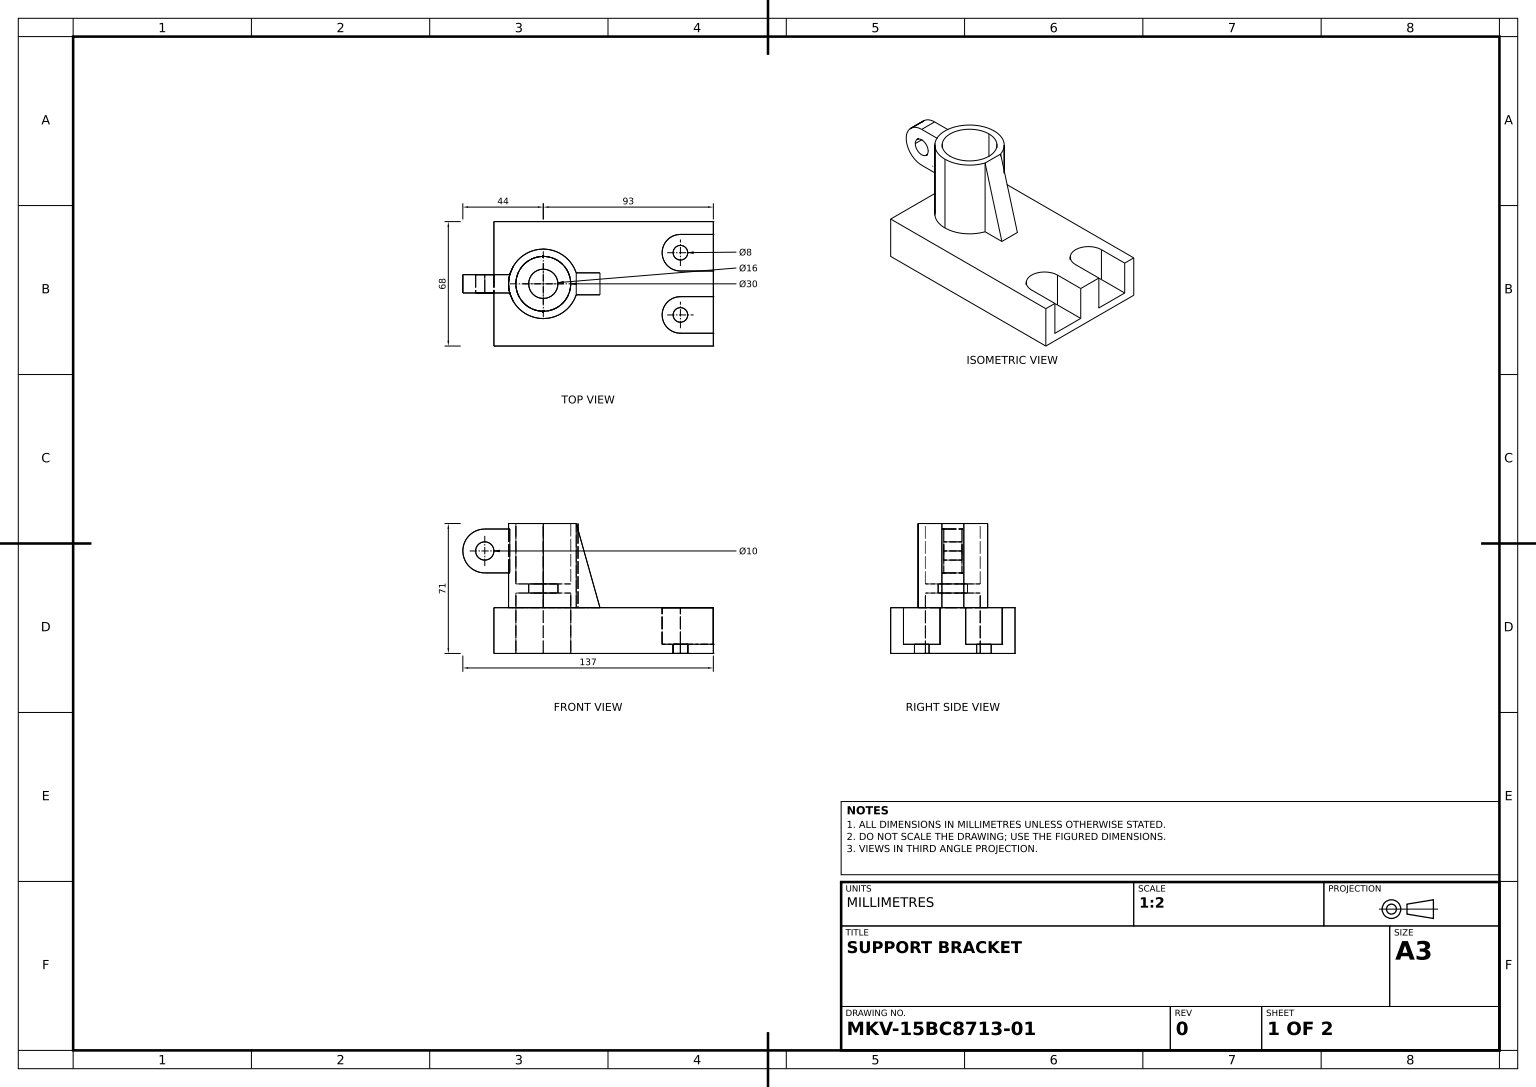
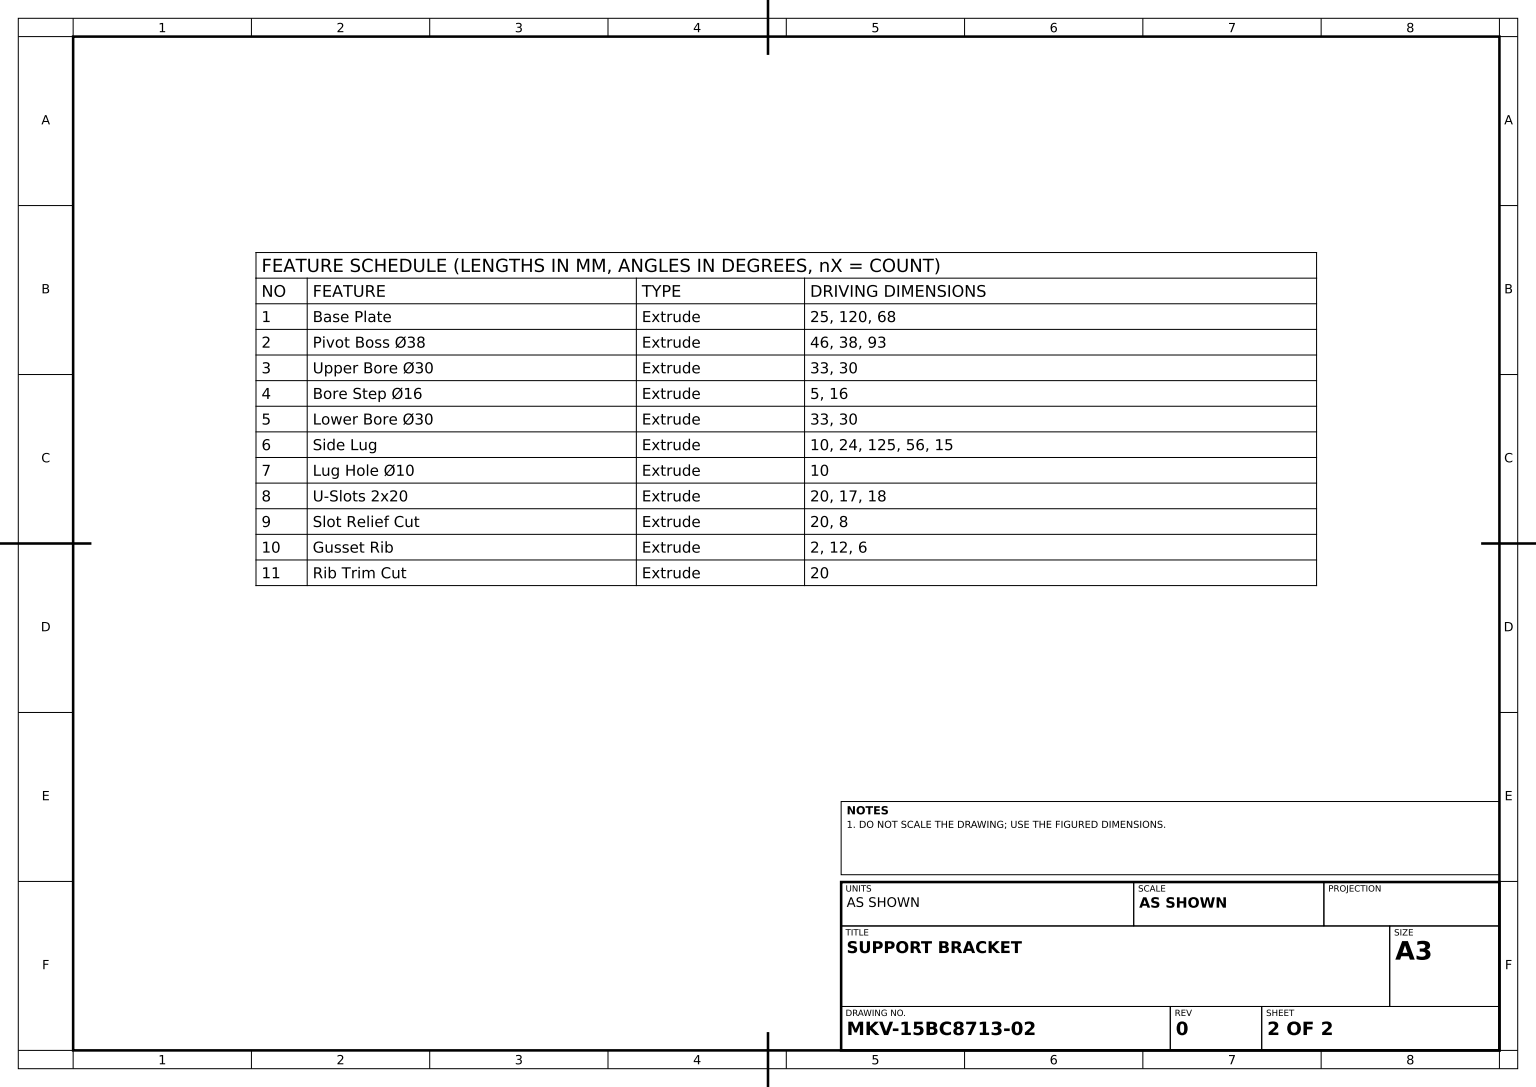
from build123d import *

# Parameters (mm, degrees)
BASE_PLATE_SKETCH_W   = 120
BASE_PLATE_SKETCH_H   = 68
BASE_PLATE_DEPTH      = 25
PIVOT_BOSS_SKETCH_R   = 19
PIVOT_BOSS_38_DEPTH   = 46
UPPER_BORE_SKETCH_R   = 15
UPPER_BORE_30_DEPTH   = 33
BORE_STEP_SKETCH_R    = 8
BORE_STEP_16_DEPTH    = 5
LOWER_BORE_SKETCH_R   = 15
LOWER_BORE_30_DEPTH   = 33
SIDE_LUG_DEPTH        = 5
LUG_HOLE_SKETCH_R     = 5
LUG_HOLE_10_DEPTH     = 10
U_SLOTS_2X20_DEPTH    = 20
SLOT_RELIEF_SKETCH_R  = 4
SLOT_RELIEF_CUT_DEPTH = 20
GUSSET_RIB_REACH      = 110.729
GUSSET_RIB_END_RADIUS = 19
GUSSET_RIB_SKETCH_W   = 12
GUSSET_RIB_SKETCH_H   = 46
RIB_TRIM_CUT_DEPTH    = 20


with BuildPart() as part:
    # Base Plate Sketch → Base Plate (new body)
    with BuildSketch(Plane(origin=(0, 0, 0), x_dir=(1, 0, 0), z_dir=(0, 1, 0))):
        Rectangle(BASE_PLATE_SKETCH_W, BASE_PLATE_SKETCH_H)
    extrude(amount=BASE_PLATE_DEPTH)

    # Pivot Boss Sketch → Pivot Boss Ø38 (add)
    with BuildSketch(Plane(origin=(0, 25, 0), x_dir=(1, 0, 0), z_dir=(0, 1, 0))):
        with Locations(Location((-33, 0, 0), (0, 0, 90))):
            Circle(PIVOT_BOSS_SKETCH_R)
    extrude(amount=PIVOT_BOSS_38_DEPTH)

    # Upper Bore Sketch → Upper Bore Ø30 (cut)
    with BuildSketch(Plane(origin=(0, 71, 0), x_dir=(1, 0, 0), z_dir=(0, 1, 0))):
        with Locations(Location((-33, 0, 0), (0, 0, 270))):
            Circle(UPPER_BORE_SKETCH_R)
    extrude(amount=-UPPER_BORE_30_DEPTH, mode=Mode.SUBTRACT)

    # Bore Step Sketch → Bore Step Ø16 (cut)
    with BuildSketch(Plane(origin=(0, 38, 0), x_dir=(1, 0, 0), z_dir=(0, 1, 0))):
        with Locations(Location((-33, 0, 0), (0, 0, 270))):
            Circle(BORE_STEP_SKETCH_R)
    extrude(amount=-BORE_STEP_16_DEPTH, mode=Mode.SUBTRACT)

    # Lower Bore Sketch → Lower Bore Ø30 (cut)
    with BuildSketch(Plane(origin=(0, 33, 0), x_dir=(1, 0, 0), z_dir=(0, 1, 0))):
        with Locations(Location((-33, 0, 0), (0, 0, 270))):
            Circle(LOWER_BORE_SKETCH_R)
    extrude(amount=-LOWER_BORE_30_DEPTH, mode=Mode.SUBTRACT)

    # Side Lug Sketch → Side Lug (add, symmetric)
    with BuildSketch(Plane.XY):
        with BuildLine():
            Line((-65, 68), (-50, 68))
            Line((-50, 68), (-50, 44))
            Line((-50, 44), (-65, 44))
            ThreePointArc((-65, 44), (-77, 56), (-65, 68))
        make_face()
    extrude(amount=SIDE_LUG_DEPTH, both=True)

    # Lug Hole Sketch → Lug Hole Ø10 (cut)
    with BuildSketch(Plane.XY.offset(5)):
        with Locations((-65, 56)):
            Circle(LUG_HOLE_SKETCH_R)
    extrude(amount=-LUG_HOLE_10_DEPTH, mode=Mode.SUBTRACT)

    # U-Slots Sketch → U-Slots 2x20 (cut)
    with BuildSketch(Plane(origin=(0, 25, 0), x_dir=(1, 0, 0), z_dir=(0, 1, 0))):
        with BuildLine():
            Line((42, 27), (60, 27))
            Line((60, 27), (60, 7))
            Line((60, 7), (42, 7))
            ThreePointArc((42, 7), (32, 17), (42, 27))
        make_face()
        with BuildLine():
            Line((42, -7), (60, -7))
            Line((60, -7), (60, -27))
            Line((60, -27), (42, -27))
            ThreePointArc((42, -27), (32, -17), (42, -7))
        make_face()
    extrude(amount=-U_SLOTS_2X20_DEPTH, mode=Mode.SUBTRACT)

    # Slot Relief Sketch → Slot Relief Cut (cut)
    with BuildSketch(Plane(origin=(0, 5, 0), x_dir=(1, 0, 0), z_dir=(0, 1, 0))):
        with Locations(Location((42, 17, 0), (0, 0, 270))):
            Circle(SLOT_RELIEF_SKETCH_R)
        with Locations(Location((42, -17, 0), (0, 0, 270))):
            Circle(SLOT_RELIEF_SKETCH_R)
    extrude(amount=-SLOT_RELIEF_CUT_DEPTH, mode=Mode.SUBTRACT)

    # Gusset Rib: up to this cylinder (the profile starts outside it)
    gusset_rib_end = Plane(origin=(-33, 48, 0), z_dir=(0, -1, 0)) * Cylinder(GUSSET_RIB_END_RADIUS, 260.458, mode=Mode.PRIVATE)
    # Gusset Rib Sketch → Gusset Rib (add, up to the surface)
    with BuildSketch(Plane(origin=(-2, 0, 0), x_dir=(0, 0, -1), z_dir=(1, 0, 0)), mode=Mode.PRIVATE) as gusset_rib_sk1:
        with Locations((0, 48)):
            Rectangle(GUSSET_RIB_SKETCH_W, GUSSET_RIB_SKETCH_H)
    gusset_rib_tool1 = extrude(gusset_rib_sk1.sketch, amount=-GUSSET_RIB_REACH, mode=Mode.PRIVATE) - gusset_rib_end
    add(gusset_rib_tool1.solids().sort_by_distance((-2, 48, 0))[0])

    # Rib Trim Sketch → Rib Trim Cut (cut)
    with BuildSketch(Plane.XY.offset(6)):
        Polygon((-14.972243623, 71), (-2, 25), (-2, 71), align=None)
    extrude(amount=-RIB_TRIM_CUT_DEPTH, mode=Mode.SUBTRACT)


solid = part.part
